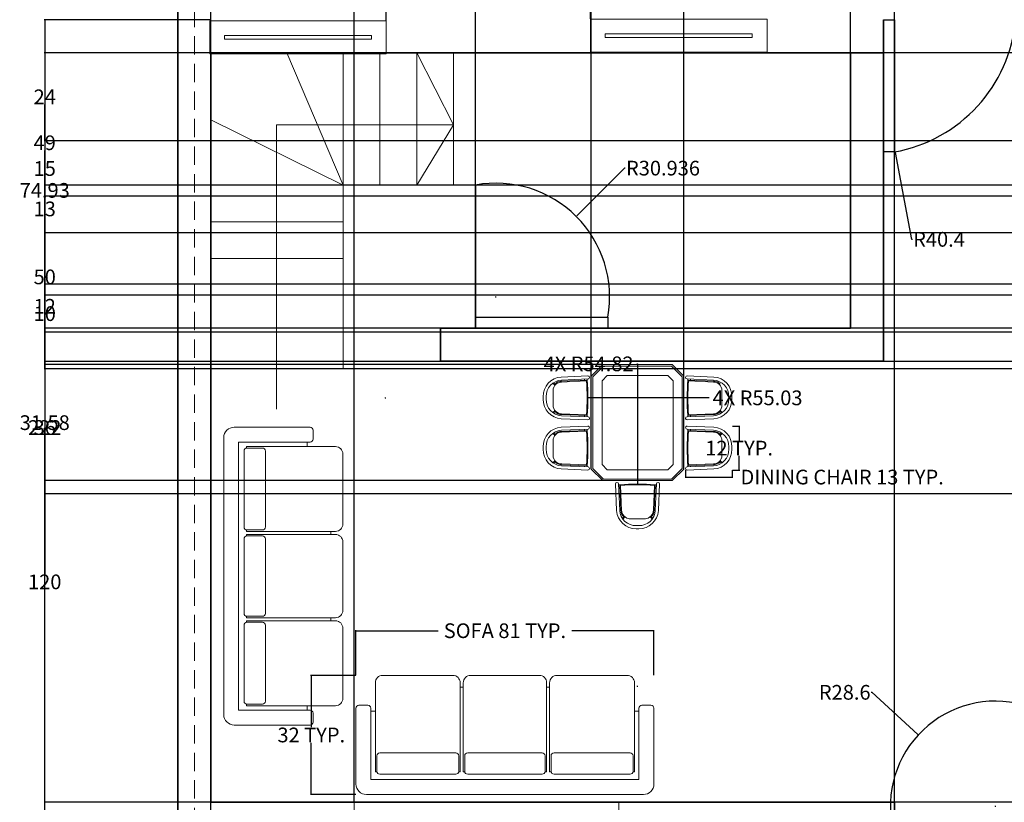
# Model space of a CAD drawing. Units: inches. Extents: x 1291 to 2095, y 532 to 1090.
# Tile 2 of 14: x 1291 to 1559, y 733 to 946. Entities that reach past the tile are written whole.
import ezdxf

# ---------------------------------------------------------------- set-up
doc = ezdxf.new("R2010")
doc.units = ezdxf.units.IN
doc.header["$MEASUREMENT"] = 0
doc.linetypes.add('HIDDEN', pattern=[0.375, 0.25, -0.125])
for name, color, linetype, lineweight in [('A-ANNO-DIMS', 2, 'Continuous', 18), ('A-DOOR', 3, 'Continuous', 25), ('A-FLOR-STRS', 7, 'Continuous', 20), ('A-FURN', 8, 'Continuous', 18), ('A-GLAZ', 4, 'Continuous', 18), ('A-WALL', 7, 'Continuous', 35), ('A-WALL-HIDN', 8, 'HIDDEN', 13)]:
    doc.layers.add(name, color=color, linetype=linetype, lineweight=lineweight)
doc.styles.get("Standard").update_dxf_attribs({"font": 'arial.ttf'})
doc.dimstyles.get("Standard").update_dxf_attribs({"dimtxt": 4, "dimasz": 0.18, "dimexe": 0.18, "dimexo": 0.0625, "dimgap": 0.09, "dimtad": 0, "dimtih": 1, "dimtoh": 1, "dimdec": 0, "dimrnd": 6, "dimzin": 0, "dimdsep": 46, "dimlunit": 3, "dimtxsty": 'Standard', "dimcen": 0.09, "dimadec": 0, "dimazin": 0, "dimtfac": 1, "dimtdec": 0, "dimtofl": 0, "dimtmove": 0, "dimatfit": 3, "dimfxl": 1, "dimtolj": 1, "dimtzin": 0, "dimarcsym": 0})

# ---------------------------------------------------------------- blocks, each defined once
blk = doc.blocks.new('A$C06FC73D7')
for p, q in [((1.93, 0.8), (0.07, 0.8)), ((0, 0.73), (0, 0.22)), ((2, 0.22), (2, 0.73)), ((0.1, 0.22), (0.1, 0.7)), ((0.1, 0.7), (1.9, 0.7)), ((0.67, 0.6637), (0.16, 0.6637)), ((1.25, 0.6637), (0.75, 0.6637)), ((1.84, 0.6637), (1.33, 0.6637)), ((1.9, 0.7), (1.9, 0.22)), ((0.13, 0.6479), (0.13, 0.05)), ((0.1404, 0.6479), (0.13, 0.6479)), ((0.14, 0.54), (0.14, 0.6437)), ((0.7, 0.6479), (0.6896, 0.6479)), ((0.69, 0.54), (0.69, 0.6437)), ((0.7, 0.05), (0.7, 0.6479)), ((0.72, 0.05), (0.72, 0.6479)), ((0.7304, 0.6479), (0.72, 0.6479)), ((0.73, 0.54), (0.73, 0.6437)), ((1.28, 0.6479), (1.2696, 0.6479)), ((1.27, 0.54), (1.27, 0.6437)), ((1.28, 0.05), (1.28, 0.6479)), ((1.3, 0.05), (1.3, 0.6479)), ((1.3104, 0.6479), (1.3, 0.6479)), ((1.31, 0.54), (1.31, 0.6437)), ((1.87, 0.6479), (1.86, 0.6479)), ((1.86, 0.54), (1.86, 0.6437)), ((1.87, 0.05), (1.87, 0.6479)), ((0.67, 0.52), (0.16, 0.52)), ((1.25, 0.52), (0.75, 0.52)), ((1.84, 0.52), (1.33, 0.52)), ((0.02, 0.2), (0.08, 0.2)), ((0.13, 0.24), (0.1, 0.24)), ((1.9, 0.24), (1.87, 0.24)), ((1.92, 0.2), (1.98, 0.2)), ((0.72, 0.08), (0.7, 0.08)), ((1.3, 0.08), (1.28, 0.08)), ((0.65, 0), (0.18, 0)), ((1.23, 0), (0.77, 0)), ((1.82, 0), (1.35, 0))]:
    blk.add_line(p, q)
for centre, radius, start, end in [((0.07, 0.73), 0.07, 90, 180), ((1.93, 0.73), 0.07, 0, 90), ((0.16, 0.6437), 0.02, 90, 180), ((0.67, 0.6437), 0.02, 0, 90), ((0.75, 0.6437), 0.02, 90, 180), ((1.25, 0.6437), 0.02, 0, 90), ((1.33, 0.6437), 0.02, 90, 180), ((1.84, 0.6437), 0.02, 0, 90), ((0.16, 0.54), 0.02, 180, 270), ((0.67, 0.54), 0.02, 270, 0), ((0.75, 0.54), 0.02, 180, 270), ((1.25, 0.54), 0.02, 270, 0), ((1.33, 0.54), 0.02, 180, 270), ((1.84, 0.54), 0.02, 270, 0), ((0.02, 0.22), 0.02, 180, 270), ((0.08, 0.22), 0.02, 270, 0), ((1.92, 0.22), 0.02, 180, 270), ((1.98, 0.22), 0.02, 270, 0), ((0.18, 0.05), 0.05, 180, 270), ((0.65, 0.05), 0.05, 270, 0), ((0.77, 0.05), 0.05, 180, 270), ((1.23, 0.05), 0.05, 270, 0), ((1.35, 0.05), 0.05, 180, 270), ((1.82, 0.05), 0.05, 270, 0)]:
    blk.add_arc(centre, radius, start, end)
blk = doc.blocks.new('A$C2BDD4447')
blk.add_blockref('A$C06FC73D7', (0, 0))
blk = doc.blocks.new('WIN-72IN')
for points in [[(0, 0), (0, 9), (72, 9), (72, 0)], [(4, 4), (4, 5), (68, 5), (68, 4)]]:
    blk.add_lwpolyline(points, close=True)
blk = doc.blocks.new('WIN-48IN')
for points in [[(0, 0), (0, 9), (48, 9), (48, 0)], [(4, 4), (4, 5), (44, 5), (44, 4)]]:
    blk.add_lwpolyline(points, close=True)
blk = doc.blocks.new('CHAIR-DINING')
for p, q in [((7.64, 10.83), (0.4, 11.13)), ((0.65, 11.13), (0.65, 10.81)), ((7.78, 10.51), (0.65, 10.8)), ((1.33, 11.1), (1.33, 10.78)), ((7.77, 10.3), (0.84, 10.59)), ((9.24, 9.6), (9.82, 10.09)), ((9.38, 9.44), (9.96, 9.93)), ((9.89, 3.77), (9.89, 8.24)), ((11.77, 5.65), (11.77, 6.32)), ((12.62, 5.64), (12.62, 6.33)), ((7.58, 1.45), (0.65, 1.16)), ((0.65, 0.84), (0.65, 1.15)), ((7.57, 1.66), (0.84, 1.38)), ((1.33, 0.87), (1.33, 1.18)), ((9.24, 2.37), (9.82, 1.88)), ((9.38, 2.53), (9.96, 2.04))]:
    blk.add_line(p, q)
for points in [[(7.68, 11.67), (0.44, 11.97, 1), (0.4, 11.13)], [(7.64, 1.14), (0.4, 0.84, 1), (0.44, 0), (7.68, 0.3)]]:
    blk.add_lwpolyline(points, format="xyb")
for centre, radius, start, end in [((55.47, 5.96), 55.03, 174.9478, 185.0066), ((7.37, 6.43), 4.41, 358.6114, 86.5609), ((7.37, 6.43), 5.25, 358.6113, 86.5608), ((55.47, 5.96), 54.82, 175.1561, 184.7886), ((7.58, 7.99), 2.52, 43.3469, 90), ((7.58, 7.99), 2.31, 0, 90), ((7.37, 5.54), 4.41, 273.4392, 1.3914), ((7.37, 5.54), 5.25, 273.4393, 1.3911), ((7.58, 3.97), 2.31, 270, 0), ((7.58, 3.97), 2.52, 270, 316.6497)]:
    blk.add_arc(centre, radius, start, end)
blk = doc.blocks.new('*D22')
at = {"layer": 'A-ANNO-DIMS', "color": 0, "lineweight": -2, "transparency": 16777216}
for p, q in [((1382.55, 767.39), (1382.55, 779.66)), ((1463.6, 767.39), (1463.6, 779.66)), ((1382.73, 779.48), (1404.87, 779.48)), ((1463.42, 779.48), (1441.27, 779.48))]:
    blk.add_line(p, q, dxfattribs=at)
at = {"layer": 'A-ANNO-DIMS', "color": 0, "transparency": 16777216}
for points in [[(1382.73, 779.51), (1382.73, 779.45), (1382.55, 779.48)], [(1463.42, 779.51), (1463.42, 779.45), (1463.6, 779.48)]]:
    blk.add_solid(points, dxfattribs=at)
at = {"layer": 'Defpoints', "color": 0, "transparency": 16777216}
for p in [(1382.55, 779.48), (1382.55, 767.33), (1463.6, 767.33)]:
    blk.add_point(p, dxfattribs=at)
at = {"layer": 'A-ANNO-DIMS', "color": 0, "transparency": 16777216, "insert": (1423.07, 779.48), "char_height": 4, "attachment_point": 5}
blk.add_mtext('\\A1;SOFA 81 TYP.', dxfattribs=at)
blk = doc.blocks.new('*D23')
at = {"layer": 'A-ANNO-DIMS', "color": 0, "lineweight": -2, "transparency": 16777216}
for p, q in [((1382.48, 767.33), (1370.21, 767.33)), ((1370.39, 767.15), (1370.39, 753.25)), ((1370.39, 735.08), (1370.39, 748.98)), ((1382.48, 734.9), (1370.21, 734.9))]:
    blk.add_line(p, q, dxfattribs=at)
at = {"layer": 'A-ANNO-DIMS', "color": 0, "transparency": 16777216}
for points in [[(1370.36, 767.15), (1370.42, 767.15), (1370.39, 767.33)], [(1370.36, 735.08), (1370.42, 735.08), (1370.39, 734.9)]]:
    blk.add_solid(points, dxfattribs=at)
at = {"layer": 'Defpoints', "color": 0, "transparency": 16777216}
for p in [(1382.55, 767.33), (1370.39, 734.9), (1382.55, 734.9)]:
    blk.add_point(p, dxfattribs=at)
at = {"layer": 'A-ANNO-DIMS', "color": 0, "transparency": 16777216, "insert": (1370.39, 751.11), "char_height": 4, "attachment_point": 5}
blk.add_mtext('\\A1;32 TYP.', dxfattribs=at)
blk = doc.blocks.new('*D24')
at = {"layer": 'A-ANNO-DIMS', "color": 0, "lineweight": -2, "transparency": 16777216}
for p, q in [((1472.2, 823.14), (1472.2, 821.12)), ((1484.89, 823.14), (1484.89, 821.12)), ((1472.38, 821.3), (1484.71, 821.3)), ((1484.89, 821.3), (1485.07, 821.3))]:
    blk.add_line(p, q, dxfattribs=at)
at = {"layer": 'A-ANNO-DIMS', "color": 0, "transparency": 16777216}
for points in [[(1472.38, 821.33), (1472.38, 821.27), (1472.2, 821.3)], [(1484.71, 821.33), (1484.71, 821.27), (1484.89, 821.3)]]:
    blk.add_solid(points, dxfattribs=at)
at = {"layer": 'Defpoints', "color": 0, "transparency": 16777216}
for p in [(1472.2, 823.2), (1484.89, 823.2), (1484.89, 821.3)]:
    blk.add_point(p, dxfattribs=at)
at = {"layer": 'A-ANNO-DIMS', "color": 0, "transparency": 16777216, "insert": (1514.82, 821.3), "char_height": 4, "attachment_point": 5}
blk.add_mtext('\\A1;DINING CHAIR 13 TYP.', dxfattribs=at)
blk = doc.blocks.new('*D25')
at = {"layer": 'A-ANNO-DIMS', "color": 0, "lineweight": -2, "transparency": 16777216}
for p, q in [((1484.95, 835.19), (1486.98, 835.19)), ((1486.8, 835.01), (1486.8, 831.29)), ((1486.8, 823.38), (1486.8, 827.09)), ((1484.95, 823.2), (1486.98, 823.2))]:
    blk.add_line(p, q, dxfattribs=at)
at = {"layer": 'A-ANNO-DIMS', "color": 0, "transparency": 16777216}
for points in [[(1486.77, 835.01), (1486.83, 835.01), (1486.8, 835.19)], [(1486.77, 823.38), (1486.83, 823.38), (1486.8, 823.2)]]:
    blk.add_solid(points, dxfattribs=at)
at = {"layer": 'Defpoints', "color": 0, "transparency": 16777216}
for p in [(1484.89, 835.19), (1486.8, 835.19), (1484.89, 823.2)]:
    blk.add_point(p, dxfattribs=at)
at = {"layer": 'A-ANNO-DIMS', "color": 0, "transparency": 16777216, "insert": (1486.8, 829.19), "char_height": 4, "attachment_point": 5}
blk.add_mtext('\\A1;12 TYP.', dxfattribs=at)
blk = doc.blocks.new('*D35')
at = {"layer": 'A-ANNO-DIMS', "color": 0, "lineweight": -2, "transparency": 16777216}
for p, q in [((1343.01, 945.78), (1297.69, 945.78)), ((1297.87, 945.6), (1297.87, 836.88)), ((1297.87, 723.96), (1297.87, 832.68)), ((1343.01, 723.78), (1297.69, 723.78))]:
    blk.add_line(p, q, dxfattribs=at)
at = {"layer": 'A-ANNO-DIMS', "color": 0, "transparency": 16777216}
for points in [[(1297.84, 945.6), (1297.9, 945.6), (1297.87, 945.78)], [(1297.84, 723.96), (1297.9, 723.96), (1297.87, 723.78)]]:
    blk.add_solid(points, dxfattribs=at)
at = {"layer": 'Defpoints', "color": 0, "transparency": 16777216}
for p in [(1297.87, 945.78), (1343.07, 945.78), (1343.07, 723.78)]:
    blk.add_point(p, dxfattribs=at)
at = {"layer": 'A-ANNO-DIMS', "color": 0, "transparency": 16777216, "insert": (1297.87, 834.78), "char_height": 4, "attachment_point": 5}
blk.add_mtext('\\A1;222', dxfattribs=at)
blk = doc.blocks.new('*D44')
at = {"layer": 'A-ANNO-DIMS', "color": 0, "lineweight": -2, "transparency": 16777216}
for p, q in [((1343.07, 579.84), (1343.07, 1087.16)), ((1343.25, 1086.98), (1451.42, 1086.98)), ((1576.43, 1086.98), (1468.26, 1086.98)), ((1576.61, 579.84), (1576.61, 1087.16))]:
    blk.add_line(p, q, dxfattribs=at)
at = {"layer": 'A-ANNO-DIMS', "color": 0, "transparency": 16777216}
for points in [[(1343.25, 1087.01), (1343.25, 1086.95), (1343.07, 1086.98)], [(1576.43, 1087.01), (1576.43, 1086.95), (1576.61, 1086.98)]]:
    blk.add_solid(points, dxfattribs=at)
at = {"layer": 'Defpoints', "color": 0, "transparency": 16777216}
for p in [(1576.61, 1086.98), (1343.07, 579.78), (1576.61, 579.78)]:
    blk.add_point(p, dxfattribs=at)
at = {"layer": 'A-ANNO-DIMS', "color": 0, "transparency": 16777216, "insert": (1459.84, 1086.98), "char_height": 4, "attachment_point": 5}
blk.add_mtext('\\A1;233.54', dxfattribs=at)
blk = doc.blocks.new('*D48')
at = {"layer": 'A-ANNO-DIMS', "color": 0, "lineweight": -2, "transparency": 16777216}
for p, q in [((1577.01, 852.78), (1297.69, 852.78)), ((1297.87, 852.6), (1297.87, 836.91)), ((1297.87, 816.96), (1297.87, 832.65)), ((1577.01, 816.78), (1297.69, 816.78))]:
    blk.add_line(p, q, dxfattribs=at)
at = {"layer": 'A-ANNO-DIMS', "color": 0, "transparency": 16777216}
for points in [[(1297.84, 852.6), (1297.9, 852.6), (1297.87, 852.78)], [(1297.84, 816.96), (1297.9, 816.96), (1297.87, 816.78)]]:
    blk.add_solid(points, dxfattribs=at)
at = {"layer": 'Defpoints', "color": 0, "transparency": 16777216}
for p in [(1297.87, 852.78), (1577.07, 852.78), (1577.07, 816.78)]:
    blk.add_point(p, dxfattribs=at)
at = {"layer": 'A-ANNO-DIMS', "color": 0, "transparency": 16777216, "insert": (1297.87, 834.78), "char_height": 4, "attachment_point": 5}
blk.add_mtext('\\A1;36', dxfattribs=at)
blk = doc.blocks.new('*D51')
at = {"layer": 'A-ANNO-DIMS', "color": 0, "lineweight": -2, "transparency": 16777216}
for p, q in [((1820.01, 852.78), (1297.69, 852.78)), ((1297.87, 852.6), (1297.87, 794.91)), ((1297.87, 732.96), (1297.87, 790.65)), ((1811.01, 732.78), (1297.69, 732.78))]:
    blk.add_line(p, q, dxfattribs=at)
at = {"layer": 'A-ANNO-DIMS', "color": 0, "transparency": 16777216}
for points in [[(1297.84, 852.6), (1297.9, 852.6), (1297.87, 852.78)], [(1297.84, 732.96), (1297.9, 732.96), (1297.87, 732.78)]]:
    blk.add_solid(points, dxfattribs=at)
at = {"layer": 'Defpoints', "color": 0, "transparency": 16777216}
for p in [(1297.87, 852.78), (1820.07, 852.78), (1811.07, 732.78)]:
    blk.add_point(p, dxfattribs=at)
at = {"layer": 'A-ANNO-DIMS', "color": 0, "transparency": 16777216, "insert": (1297.87, 792.78), "char_height": 4, "attachment_point": 5}
blk.add_mtext('\\A1;120', dxfattribs=at)
blk = doc.blocks.new('*D53')
at = {"layer": 'A-ANNO-DIMS', "color": 0, "lineweight": -2, "transparency": 16777216}
for p, q in [((1517, 936.78), (1297.69, 936.78)), ((1297.87, 936.6), (1297.87, 901.45)), ((1297.87, 862.03), (1297.87, 897.18)), ((1517, 861.85), (1297.69, 861.85))]:
    blk.add_line(p, q, dxfattribs=at)
at = {"layer": 'A-ANNO-DIMS', "color": 0, "transparency": 16777216}
for points in [[(1297.84, 936.6), (1297.9, 936.6), (1297.87, 936.78)], [(1297.84, 862.03), (1297.9, 862.03), (1297.87, 861.85)]]:
    blk.add_solid(points, dxfattribs=at)
at = {"layer": 'Defpoints', "color": 0, "transparency": 16777216}
for p in [(1297.87, 936.78), (1517.07, 936.78), (1517.07, 861.85)]:
    blk.add_point(p, dxfattribs=at)
at = {"layer": 'A-ANNO-DIMS', "color": 0, "transparency": 16777216, "insert": (1297.87, 899.32), "char_height": 4, "attachment_point": 5}
blk.add_mtext('\\A1;74.93', dxfattribs=at)
blk = doc.blocks.new('*D54')
at = {"layer": 'A-ANNO-DIMS', "color": 0, "lineweight": -2, "transparency": 16777216}
for p, q in [((1415.07, 861.91), (1415.07, 1087.16)), ((1415.25, 1086.98), (1461.77, 1086.98)), ((1516.89, 1086.98), (1470.37, 1086.98)), ((1517.07, 861.91), (1517.07, 1087.16))]:
    blk.add_line(p, q, dxfattribs=at)
at = {"layer": 'A-ANNO-DIMS', "color": 0, "transparency": 16777216}
for points in [[(1415.25, 1087.01), (1415.25, 1086.95), (1415.07, 1086.98)], [(1516.89, 1087.01), (1516.89, 1086.95), (1517.07, 1086.98)]]:
    blk.add_solid(points, dxfattribs=at)
at = {"layer": 'Defpoints', "color": 0, "transparency": 16777216}
for p in [(1517.07, 1086.98), (1415.07, 861.85), (1517.07, 861.85)]:
    blk.add_point(p, dxfattribs=at)
at = {"layer": 'A-ANNO-DIMS', "color": 0, "transparency": 16777216, "insert": (1466.07, 1086.98), "char_height": 4, "attachment_point": 5}
blk.add_mtext('\\A1;102', dxfattribs=at)
blk = doc.blocks.new('*D56')
at = {"layer": 'A-ANNO-DIMS', "color": 0, "lineweight": -2, "transparency": 16777216}
for p, q in [((1868.01, 936.78), (1297.69, 936.78)), ((1297.87, 936.6), (1297.87, 914.41)), ((1297.87, 887.96), (1297.87, 910.15)), ((1868.01, 887.78), (1297.69, 887.78))]:
    blk.add_line(p, q, dxfattribs=at)
at = {"layer": 'A-ANNO-DIMS', "color": 0, "transparency": 16777216}
for points in [[(1297.84, 936.6), (1297.9, 936.6), (1297.87, 936.78)], [(1297.84, 887.96), (1297.9, 887.96), (1297.87, 887.78)]]:
    blk.add_solid(points, dxfattribs=at)
at = {"layer": 'Defpoints', "color": 0, "transparency": 16777216}
for p in [(1297.87, 936.78), (1868.07, 936.78), (1868.07, 887.78)]:
    blk.add_point(p, dxfattribs=at)
at = {"layer": 'A-ANNO-DIMS', "color": 0, "transparency": 16777216, "insert": (1297.87, 912.28), "char_height": 4, "attachment_point": 5}
blk.add_mtext('\\A1;49', dxfattribs=at)
blk = doc.blocks.new('*D57')
at = {"layer": 'A-ANNO-DIMS', "color": 0, "lineweight": -2, "transparency": 16777216}
for p, q in [((1973.01, 900.78), (1297.69, 900.78)), ((1297.87, 900.6), (1297.87, 896.41)), ((1297.87, 887.96), (1297.87, 892.15)), ((1973.01, 887.78), (1297.69, 887.78))]:
    blk.add_line(p, q, dxfattribs=at)
at = {"layer": 'A-ANNO-DIMS', "color": 0, "transparency": 16777216}
for points in [[(1297.84, 900.6), (1297.9, 900.6), (1297.87, 900.78)], [(1297.84, 887.96), (1297.9, 887.96), (1297.87, 887.78)]]:
    blk.add_solid(points, dxfattribs=at)
at = {"layer": 'Defpoints', "color": 0, "transparency": 16777216}
for p in [(1297.87, 900.78), (1973.07, 900.78), (1973.07, 887.78)]:
    blk.add_point(p, dxfattribs=at)
at = {"layer": 'A-ANNO-DIMS', "color": 0, "transparency": 16777216, "insert": (1297.87, 894.28), "char_height": 4, "attachment_point": 5}
blk.add_mtext('\\A1;13', dxfattribs=at)
blk = doc.blocks.new('*D59')
at = {"layer": 'A-ANNO-DIMS', "color": 0, "lineweight": -2, "transparency": 16777216}
for p, q in [((2009.01, 900.78), (1297.69, 900.78)), ((1297.87, 900.6), (1297.87, 877.91)), ((1297.87, 850.96), (1297.87, 873.65)), ((2009.01, 850.78), (1297.69, 850.78))]:
    blk.add_line(p, q, dxfattribs=at)
at = {"layer": 'A-ANNO-DIMS', "color": 0, "transparency": 16777216}
for points in [[(1297.84, 900.6), (1297.9, 900.6), (1297.87, 900.78)], [(1297.84, 850.96), (1297.9, 850.96), (1297.87, 850.78)]]:
    blk.add_solid(points, dxfattribs=at)
at = {"layer": 'Defpoints', "color": 0, "transparency": 16777216}
for p in [(1297.87, 900.78), (2009.07, 900.78), (2009.07, 850.78)]:
    blk.add_point(p, dxfattribs=at)
at = {"layer": 'A-ANNO-DIMS', "color": 0, "transparency": 16777216, "insert": (1297.87, 875.78), "char_height": 4, "attachment_point": 5}
blk.add_mtext('\\A1;50', dxfattribs=at)
blk = doc.blocks.new('*D60')
at = {"layer": 'A-ANNO-DIMS', "color": 0, "lineweight": -2, "transparency": 16777216}
for p, q in [((2045.01, 870.78), (1297.69, 870.78)), ((1297.87, 870.6), (1297.87, 867.91)), ((1297.87, 860.96), (1297.87, 863.65)), ((2045.01, 860.78), (1297.69, 860.78))]:
    blk.add_line(p, q, dxfattribs=at)
at = {"layer": 'A-ANNO-DIMS', "color": 0, "transparency": 16777216}
for points in [[(1297.84, 870.6), (1297.9, 870.6), (1297.87, 870.78)], [(1297.84, 860.96), (1297.9, 860.96), (1297.87, 860.78)]]:
    blk.add_solid(points, dxfattribs=at)
at = {"layer": 'Defpoints', "color": 0, "transparency": 16777216}
for p in [(1297.87, 870.78), (2045.07, 870.78), (2045.07, 860.78)]:
    blk.add_point(p, dxfattribs=at)
at = {"layer": 'A-ANNO-DIMS', "color": 0, "transparency": 16777216, "insert": (1297.87, 865.78), "char_height": 4, "attachment_point": 5}
blk.add_mtext('\\A1;10', dxfattribs=at)
blk = doc.blocks.new('*D61')
at = {"layer": 'A-ANNO-DIMS', "color": 0, "lineweight": -2, "transparency": 16777216}
for p, q in [((1343.07, 732.84), (1343.07, 1087.16)), ((1343.25, 1086.98), (1355.7, 1086.98)), ((1381.84, 1086.98), (1369.4, 1086.98)), ((1382.02, 732.91), (1382.02, 1087.16))]:
    blk.add_line(p, q, dxfattribs=at)
at = {"layer": 'A-ANNO-DIMS', "color": 0, "transparency": 16777216}
for points in [[(1343.25, 1087.01), (1343.25, 1086.95), (1343.07, 1086.98)], [(1381.84, 1087.01), (1381.84, 1086.95), (1382.02, 1086.98)]]:
    blk.add_solid(points, dxfattribs=at)
at = {"layer": 'Defpoints', "color": 0, "transparency": 16777216}
for p in [(1382.02, 1086.98), (1343.07, 732.78), (1382.02, 732.85)]:
    blk.add_point(p, dxfattribs=at)
at = {"layer": 'A-ANNO-DIMS', "color": 0, "transparency": 16777216, "insert": (1362.55, 1086.98), "char_height": 4, "attachment_point": 5}
blk.add_mtext('\\A1;38.95', dxfattribs=at)
blk = doc.blocks.new('*D63')
at = {"layer": 'A-ANNO-DIMS', "color": 0, "lineweight": -2, "transparency": 16777216}
for p, q in [((1529.07, 723.84), (1529.07, 1087.16)), ((1529.25, 1086.98), (1544.12, 1086.98)), ((1564.89, 1086.98), (1550.03, 1086.98)), ((1565.07, 723.84), (1565.07, 1087.16))]:
    blk.add_line(p, q, dxfattribs=at)
at = {"layer": 'A-ANNO-DIMS', "color": 0, "transparency": 16777216}
for points in [[(1529.25, 1087.01), (1529.25, 1086.95), (1529.07, 1086.98)], [(1564.89, 1087.01), (1564.89, 1086.95), (1565.07, 1086.98)]]:
    blk.add_solid(points, dxfattribs=at)
at = {"layer": 'Defpoints', "color": 0, "transparency": 16777216}
for p in [(1565.07, 1086.98), (1529.07, 723.78), (1565.07, 723.78)]:
    blk.add_point(p, dxfattribs=at)
at = {"layer": 'A-ANNO-DIMS', "color": 0, "transparency": 16777216, "insert": (1547.07, 1086.98), "char_height": 4, "attachment_point": 5}
blk.add_mtext('\\A1;36', dxfattribs=at)
blk = doc.blocks.new('*D69')
at = {"layer": 'A-ANNO-DIMS', "color": 0, "lineweight": -2, "transparency": 16777216}
for p, q in [((1390.8, 945.53), (1390.8, 1087.16)), ((1390.98, 1086.98), (1411.75, 1086.98)), ((1446.2, 1086.98), (1425.43, 1086.98)), ((1446.38, 945.99), (1446.38, 1087.16))]:
    blk.add_line(p, q, dxfattribs=at)
at = {"layer": 'A-ANNO-DIMS', "color": 0, "transparency": 16777216}
for points in [[(1390.98, 1087.01), (1390.98, 1086.95), (1390.8, 1086.98)], [(1446.2, 1087.01), (1446.2, 1086.95), (1446.38, 1086.98)]]:
    blk.add_solid(points, dxfattribs=at)
at = {"layer": 'Defpoints', "color": 0, "transparency": 16777216}
for p in [(1446.38, 1086.98), (1446.38, 945.92), (1390.8, 945.47)]:
    blk.add_point(p, dxfattribs=at)
at = {"layer": 'A-ANNO-DIMS', "color": 0, "transparency": 16777216, "insert": (1418.59, 1086.98), "char_height": 4, "attachment_point": 5}
blk.add_mtext('\\A1;55.58', dxfattribs=at)
blk = doc.blocks.new('*D78')
at = {"layer": 'A-ANNO-DIMS', "color": 0, "lineweight": -2, "transparency": 16777216}
for p, q in [((1562.01, 936.78), (1297.69, 936.78)), ((1297.87, 936.6), (1297.87, 926.88)), ((1297.87, 912.96), (1297.87, 922.68)), ((1562.01, 912.78), (1297.69, 912.78))]:
    blk.add_line(p, q, dxfattribs=at)
at = {"layer": 'A-ANNO-DIMS', "color": 0, "transparency": 16777216}
for points in [[(1297.84, 936.6), (1297.9, 936.6), (1297.87, 936.78)], [(1297.84, 912.96), (1297.9, 912.96), (1297.87, 912.78)]]:
    blk.add_solid(points, dxfattribs=at)
at = {"layer": 'Defpoints', "color": 0, "transparency": 16777216}
for p in [(1297.87, 936.78), (1562.07, 936.78), (1562.07, 912.78)]:
    blk.add_point(p, dxfattribs=at)
at = {"layer": 'A-ANNO-DIMS', "color": 0, "transparency": 16777216, "insert": (1297.87, 924.78), "char_height": 4, "attachment_point": 5}
blk.add_mtext('\\A1;24', dxfattribs=at)
blk = doc.blocks.new('*D80')
at = {"layer": 'A-ANNO-DIMS', "color": 0, "lineweight": -2, "transparency": 16777216}
for p, q in [((1670.01, 912.78), (1297.69, 912.78)), ((1297.87, 912.6), (1297.87, 907.41)), ((1297.87, 897.96), (1297.87, 903.15)), ((1670.01, 897.78), (1297.69, 897.78))]:
    blk.add_line(p, q, dxfattribs=at)
at = {"layer": 'A-ANNO-DIMS', "color": 0, "transparency": 16777216}
for points in [[(1297.84, 912.6), (1297.9, 912.6), (1297.87, 912.78)], [(1297.84, 897.96), (1297.9, 897.96), (1297.87, 897.78)]]:
    blk.add_solid(points, dxfattribs=at)
at = {"layer": 'Defpoints', "color": 0, "transparency": 16777216}
for p in [(1297.87, 912.78), (1670.07, 912.78), (1670.07, 897.78)]:
    blk.add_point(p, dxfattribs=at)
at = {"layer": 'A-ANNO-DIMS', "color": 0, "transparency": 16777216, "insert": (1297.87, 905.28), "char_height": 4, "attachment_point": 5}
blk.add_mtext('\\A1;15', dxfattribs=at)
blk = doc.blocks.new('*D81')
at = {"layer": 'A-ANNO-DIMS', "color": 0, "lineweight": -2, "transparency": 16777216}
for p, q in [((1577.01, 873.78), (1297.69, 873.78)), ((1297.87, 873.6), (1297.87, 869.88)), ((1297.87, 861.96), (1297.87, 865.68)), ((1577.01, 861.78), (1297.69, 861.78))]:
    blk.add_line(p, q, dxfattribs=at)
at = {"layer": 'A-ANNO-DIMS', "color": 0, "transparency": 16777216}
for points in [[(1297.84, 873.6), (1297.9, 873.6), (1297.87, 873.78)], [(1297.84, 861.96), (1297.9, 861.96), (1297.87, 861.78)]]:
    blk.add_solid(points, dxfattribs=at)
at = {"layer": 'Defpoints', "color": 0, "transparency": 16777216}
for p in [(1297.87, 873.78), (1577.07, 873.78), (1577.07, 861.78)]:
    blk.add_point(p, dxfattribs=at)
at = {"layer": 'A-ANNO-DIMS', "color": 0, "transparency": 16777216, "insert": (1297.87, 867.78), "char_height": 4, "attachment_point": 5}
blk.add_mtext('\\A1;12', dxfattribs=at)
blk = doc.blocks.new('*D82')
at = {"layer": 'A-ANNO-DIMS', "color": 0, "lineweight": -2, "transparency": 16777216}
for p, q in [((1446.55, 823.54), (1446.55, 1087.16)), ((1446.73, 1086.98), (1450.72, 1086.98)), ((1471.56, 1086.98), (1467.57, 1086.98)), ((1471.74, 823.54), (1471.74, 1087.16))]:
    blk.add_line(p, q, dxfattribs=at)
at = {"layer": 'A-ANNO-DIMS', "color": 0, "transparency": 16777216}
for points in [[(1446.73, 1087.01), (1446.73, 1086.95), (1446.55, 1086.98)], [(1471.56, 1087.01), (1471.56, 1086.95), (1471.74, 1086.98)]]:
    blk.add_solid(points, dxfattribs=at)
at = {"layer": 'Defpoints', "color": 0, "transparency": 16777216}
for p in [(1471.74, 1086.98), (1446.55, 823.47), (1471.74, 823.47)]:
    blk.add_point(p, dxfattribs=at)
at = {"layer": 'A-ANNO-DIMS', "color": 0, "transparency": 16777216, "insert": (1459.15, 1086.98), "char_height": 4, "attachment_point": 5}
blk.add_mtext('\\A1;25.196', dxfattribs=at)
blk = doc.blocks.new('*D83')
at = {"layer": 'A-ANNO-DIMS', "color": 0, "lineweight": -2, "transparency": 16777216}
for p, q in [((1449.63, 851.9), (1297.69, 851.9)), ((1297.87, 851.72), (1297.87, 838.25)), ((1297.87, 820.5), (1297.87, 833.98)), ((1449.63, 820.32), (1297.69, 820.32))]:
    blk.add_line(p, q, dxfattribs=at)
at = {"layer": 'A-ANNO-DIMS', "color": 0, "transparency": 16777216}
for points in [[(1297.84, 851.72), (1297.9, 851.72), (1297.87, 851.9)], [(1297.84, 820.5), (1297.9, 820.5), (1297.87, 820.32)]]:
    blk.add_solid(points, dxfattribs=at)
at = {"layer": 'Defpoints', "color": 0, "transparency": 16777216}
for p in [(1297.87, 851.9), (1449.7, 851.9), (1449.7, 820.32)]:
    blk.add_point(p, dxfattribs=at)
at = {"layer": 'A-ANNO-DIMS', "color": 0, "transparency": 16777216, "insert": (1297.87, 836.11), "char_height": 4, "attachment_point": 5}
blk.add_mtext('\\A1;31.58', dxfattribs=at)
blk = doc.blocks.new('*D88')
at = {"layer": 'A-ANNO-DIMS', "color": 0, "lineweight": -2, "transparency": 16777216}
for p, q in [((1455.6, 905.38), (1442.61, 892.37)), ((1455.78, 905.38), (1455.6, 905.38)), ((1420.54, 870.35), (1420.72, 870.35)), ((1420.63, 870.26), (1420.63, 870.44))]:
    blk.add_line(p, q, dxfattribs=at)
at = {"layer": 'A-ANNO-DIMS', "color": 0, "transparency": 16777216}
blk.add_solid([(1442.59, 892.39), (1442.63, 892.35), (1442.48, 892.24)], dxfattribs=at)
at = {"layer": 'Defpoints', "color": 0, "transparency": 16777216}
for p in [(1442.48, 892.24), (1420.63, 870.35)]:
    blk.add_point(p, dxfattribs=at)
at = {"layer": 'A-ANNO-DIMS', "color": 0, "transparency": 16777216, "insert": (1466.08, 905.38), "char_height": 4, "attachment_point": 5}
blk.add_mtext('\\A1;R30.936', dxfattribs=at)
blk = doc.blocks.new('*D89')
at = {"layer": 'A-ANNO-DIMS', "color": 0, "lineweight": -2, "transparency": 16777216}
for p, q in [((1522.71, 762.72), (1522.89, 762.72)), ((1522.89, 762.72), (1535.38, 751.22)), ((1556.46, 731.72), (1556.64, 731.72)), ((1556.55, 731.63), (1556.55, 731.81))]:
    blk.add_line(p, q, dxfattribs=at)
at = {"layer": 'A-ANNO-DIMS', "color": 0, "transparency": 16777216}
blk.add_solid([(1535.4, 751.24), (1535.36, 751.2), (1535.51, 751.1)], dxfattribs=at)
at = {"layer": 'Defpoints', "color": 0, "transparency": 16777216}
for p in [(1535.51, 751.1), (1556.55, 731.72)]:
    blk.add_point(p, dxfattribs=at)
at = {"layer": 'A-ANNO-DIMS', "color": 0, "transparency": 16777216, "insert": (1515.52, 762.72), "char_height": 4, "attachment_point": 5}
blk.add_mtext('\\A1;R28.6', dxfattribs=at)
blk = doc.blocks.new('*D90')
at = {"layer": 'A-ANNO-DIMS', "color": 0, "lineweight": -2, "transparency": 16777216}
for p, q in [((1521.76, 949.52), (1521.94, 949.52)), ((1521.85, 949.43), (1521.85, 949.61)), ((1533.8, 886), (1529.35, 909.64)), ((1533.98, 886), (1533.8, 886))]:
    blk.add_line(p, q, dxfattribs=at)
at = {"layer": 'A-ANNO-DIMS', "color": 0, "transparency": 16777216}
blk.add_solid([(1529.38, 909.65), (1529.32, 909.63), (1529.32, 909.82)], dxfattribs=at)
at = {"layer": 'Defpoints', "color": 0, "transparency": 16777216}
for p in [(1521.85, 949.52), (1529.32, 909.82)]:
    blk.add_point(p, dxfattribs=at)
at = {"layer": 'A-ANNO-DIMS', "color": 0, "transparency": 16777216, "insert": (1541.17, 886), "char_height": 4, "attachment_point": 5}
blk.add_mtext('\\A1;R40.4', dxfattribs=at)
blk = doc.blocks.new('*D92')
at = {"layer": 'A-ANNO-DIMS', "color": 0, "lineweight": -2, "transparency": 16777216}
for p, q in [((1390.52, 842.82), (1390.7, 842.82)), ((1390.61, 842.73), (1390.61, 842.91)), ((1478.66, 842.86), (1445.82, 842.84))]:
    blk.add_line(p, q, dxfattribs=at)
at = {"layer": 'A-ANNO-DIMS', "color": 0, "transparency": 16777216}
blk.add_solid([(1445.82, 842.88), (1445.82, 842.82), (1445.64, 842.84)], dxfattribs=at)
at = {"layer": 'Defpoints', "color": 0, "transparency": 16777216}
for p in [(1390.61, 842.82), (1445.64, 842.84)]:
    blk.add_point(p, dxfattribs=at)
at = {"layer": 'A-ANNO-DIMS', "color": 0, "transparency": 16777216, "insert": (1491.8, 842.86), "char_height": 4, "attachment_point": 5}
blk.add_mtext('\\A1;4X R55.03', dxfattribs=at)
blk = doc.blocks.new('*D93')
at = {"layer": 'A-ANNO-DIMS', "color": 0, "lineweight": -2, "transparency": 16777216}
for p, q in [((1458.95, 852.11), (1459.13, 852.11)), ((1459.13, 852.11), (1459.15, 819.39)), ((1459.08, 764.39), (1459.26, 764.39)), ((1459.17, 764.3), (1459.17, 764.48))]:
    blk.add_line(p, q, dxfattribs=at)
at = {"layer": 'A-ANNO-DIMS', "color": 0, "transparency": 16777216}
blk.add_solid([(1459.18, 819.39), (1459.12, 819.39), (1459.15, 819.21)], dxfattribs=at)
at = {"layer": 'Defpoints', "color": 0, "transparency": 16777216}
for p in [(1459.15, 819.21), (1459.17, 764.39)]:
    blk.add_point(p, dxfattribs=at)
at = {"layer": 'A-ANNO-DIMS', "color": 0, "transparency": 16777216, "insert": (1445.84, 852.11), "char_height": 4, "attachment_point": 5}
blk.add_mtext('\\A1;4X R54.82', dxfattribs=at)

msp = doc.modelspace()

# ---------------------------------------------------------------- linework, layer by layer
at = {"layer": 'A-DOOR'}
for points in [[(1526.0658, 945.7707), (1529.0658, 945.7707), (1529.0658, 909.7707), (1526.0658, 909.7707)], [(1451.0735, 864.8516), (1451.0735, 861.8516), (1415.0735, 861.8516), (1415.0735, 864.8516)]]:
    msp.add_lwpolyline(points, close=True, dxfattribs=at)
for centre, radius, start, end in [((1521.8491, 949.5186), 40.3978, 280.290544, 354.690499), ((1420.6291, 870.3469), 30.9364, 349.767963, 100.345385), ((1556.5498, 731.7195), 28.6002, 78.580328, 196.116311)]:
    msp.add_arc(centre, radius, start, end, dxfattribs=at)
at = {"layer": 'A-FLOR-STRS'}
for p, q in [((1379.0735, 900.7804), (1363.7205, 936.7804)), ((1379.0735, 936.7804), (1379.0735, 850.7804)), ((1389.0735, 936.7804), (1389.0735, 900.7804)), ((1399.0735, 936.7804), (1399.0735, 900.7804)), ((1409.0735, 917.193), (1399.0735, 936.7804)), ((1409.0735, 936.7804), (1409.0735, 900.7804)), ((1415.0735, 936.7804), (1415.0735, 900.7804)), ((1379.0735, 900.7804), (1343.0735, 918.5024)), ((1360.9052, 839.8148), (1360.9052, 917.193)), ((1360.9052, 917.193), (1409.0735, 917.193)), ((1409.0735, 917.193), (1399.0735, 900.7804)), ((1415.0735, 900.7804), (1343.0735, 900.7804)), ((1379.0735, 890.7804), (1343.0735, 890.7804)), ((1379.0735, 880.7804), (1343.0735, 880.7804)), ((1379.0735, 870.7804), (1343.0735, 870.7804)), ((1379.0735, 860.7804), (1343.0735, 860.7804)), ((1379.0735, 850.7804), (1343.0735, 850.7804))]:
    msp.add_line(p, q, dxfattribs=at)
at = {"layer": 'A-FURN'}
for p, q in [((1436.7019, 846.3016), (1436.1232, 846.795)), ((1436.8382, 846.4613), (1436.2595, 846.9548)), ((1438.3016, 847.3741), (1445.4359, 847.6703)), ((1438.3147, 847.1643), (1445.2392, 847.4522)), ((1438.4453, 847.6941), (1445.6799, 847.9947)), ((1444.7499, 847.9649), (1444.7499, 847.6506)), ((1445.4351, 847.9947), (1445.4351, 847.6791)), ((1479.8459, 847.6941), (1472.6113, 847.9947)), ((1479.9895, 847.3741), (1472.8553, 847.6703)), ((1472.8561, 847.9947), (1472.8561, 847.6791)), ((1479.9765, 847.1643), (1473.052, 847.4522)), ((1473.5412, 847.9649), (1473.5412, 847.6506)), ((1436.1942, 840.6348), (1436.1942, 845.1016)), ((1482.097, 840.6348), (1482.097, 845.1016)), ((1433.4669, 842.5039), (1433.4669, 843.1947)), ((1434.3072, 842.5146), (1434.3072, 843.185)), ((1483.984, 842.5146), (1483.984, 843.185)), ((1484.8242, 842.5039), (1484.8242, 843.1947)), ((1436.7019, 839.3983), (1436.1232, 838.9046)), ((1436.8382, 839.2385), (1436.2595, 838.745)), ((1438.5099, 838.5273), (1445.2438, 838.2474)), ((1479.7813, 838.5273), (1473.0474, 838.2474)), ((1481.453, 839.2385), (1482.0317, 838.745)), ((1481.5893, 839.3983), (1482.168, 838.9046)), ((1438.5059, 838.3173), (1445.4357, 838.0293)), ((1444.7499, 837.7349), (1444.7499, 838.049)), ((1445.4351, 837.7049), (1445.4351, 838.0207)), ((1479.7852, 838.3173), (1472.8555, 838.0293)), ((1472.8561, 837.7049), (1472.8561, 838.0207)), ((1473.5412, 837.7349), (1473.5412, 838.049)), ((1454.3014, 812.2219), (1454.0008, 819.4565)), ((1454.0008, 819.2117), (1454.3163, 819.2117)), ((1454.0306, 818.5266), (1454.3449, 818.5266)), ((1454.6214, 812.0783), (1454.3252, 819.2126)), ((1454.8312, 812.0913), (1454.5433, 819.0158)), ((1463.4682, 812.2866), (1463.7481, 819.0204)), ((1463.6781, 812.2826), (1463.9662, 819.2123)), ((1464.2606, 818.5266), (1463.9465, 818.5266)), ((1464.2906, 819.2117), (1463.9748, 819.2117)), ((1455.5341, 810.6148), (1455.0407, 810.0361)), ((1455.6939, 810.4786), (1455.2005, 809.8999)), ((1461.3607, 809.9708), (1456.8939, 809.9708)), ((1462.5972, 810.4786), (1463.0909, 809.8999)), ((1462.757, 810.6148), (1463.2504, 810.0361)), ((1459.4916, 807.2436), (1458.8008, 807.2436)), ((1459.4809, 808.0839), (1458.8105, 808.0839))]:
    msp.add_line(p, q, dxfattribs=at)
for points in [[(1471.7436, 823.4737), (1471.7436, 848.7533), (1468.5941, 851.9028), (1449.6971, 851.9028), (1446.5476, 848.7533), (1446.5476, 823.4737), (1449.6971, 820.3242), (1468.5941, 820.3242)], [(1471.3237, 848.5793), (1471.3237, 823.6352), (1468.4327, 820.7441), (1449.8833, 820.7441), (1446.9862, 823.6413), (1446.9675, 848.5793), (1449.8711, 851.4829), (1468.4203, 851.4829)], [(1468.8041, 847.5357), (1468.8041, 824.6913), (1467.3765, 823.2638), (1450.9147, 823.2638), (1449.4871, 824.6913), (1449.4871, 847.5357), (1450.9147, 848.9633), (1467.3765, 848.9633)]]:
    msp.add_lwpolyline(points, close=True, dxfattribs=at)
for points in [[(1445.6799, 847.9945, 1), (1445.645, 848.834), (1438.4018, 848.5329)], [(1479.8894, 848.5329), (1472.6462, 848.834, 1), (1472.6113, 847.9945)], [(1438.4018, 837.1669), (1445.645, 836.8658, 1), (1445.6799, 837.7049), (1438.4453, 838.0058)], [(1479.8459, 838.0058), (1472.6113, 837.7049, 1), (1472.6462, 836.8658), (1479.8894, 837.1669)], [(1454.001, 819.4565, 1), (1453.1615, 819.4217), (1453.4626, 812.1784)], [(1464.8286, 812.1784), (1465.1296, 819.4217, 1), (1464.2906, 819.4565), (1463.9897, 812.2219)]]:
    msp.add_lwpolyline(points, format="xyb", dxfattribs=at)
for centre, radius, start, end in [((1438.7161, 843.2921), 5.2501, 93.439216, 181.388744), ((1438.7161, 843.2921), 4.4102, 93.439136, 181.388601), ((1438.5062, 844.8606), 2.3119, 90, 180), ((1438.5062, 844.8606), 2.5218, 90, 136.653148), ((1390.6114, 842.8234), 54.8236, 355.211394, 4.843878), ((1390.6114, 842.8234), 55.0335, 354.993413, 5.052231), ((1527.6798, 842.8234), 55.0335, 174.947769, 185.006587), ((1527.6798, 842.8234), 54.8236, 175.156122, 184.788606), ((1479.785, 844.8606), 2.5218, 43.346852, 90), ((1479.785, 844.8606), 2.3119, 0, 90), ((1479.5751, 843.2921), 4.4102, 358.611399, 86.560864), ((1479.5751, 843.2921), 5.2501, 358.611256, 86.560784), ((1438.7161, 842.4075), 5.25, 178.608948, 266.560743), ((1438.7161, 842.4075), 4.4101, 178.608646, 266.560815), ((1479.5751, 842.4075), 4.4101, 273.439185, 1.391354), ((1479.5751, 842.4075), 5.25, 273.439257, 1.391052), ((1438.5062, 840.8393), 2.3119, 180, 270), ((1438.5062, 840.8393), 2.5219, 223.350321, 270), ((1479.785, 840.8393), 2.3119, 270, 0), ((1479.785, 840.8393), 2.5219, 270, 316.649679), ((1459.172, 764.388), 55.0335, 84.993413, 95.052231), ((1459.172, 764.388), 54.8236, 85.211394, 94.843878), ((1458.7034, 812.4928), 5.2501, 183.439216, 271.388744), ((1458.7034, 812.4928), 4.4102, 183.439136, 271.388601), ((1457.1349, 812.2828), 2.5218, 180, 226.653148), ((1457.1349, 812.2828), 2.3119, 180, 270), ((1459.588, 812.4928), 5.25, 268.608948, 356.560743), ((1459.588, 812.4928), 4.4101, 268.608646, 356.560815), ((1461.1562, 812.2828), 2.3119, 270, 0), ((1461.1562, 812.2828), 2.5219, 313.350321, 0)]:
    msp.add_arc(centre, radius, start, end, dxfattribs=at)
at = {"layer": 'A-WALL'}
for p, q in [((1334.0735, 1050.7804), (1334.0735, 570.7804)), ((1526.0735, 936.7804), (1526.0735, 945.7804)), ((1526.0735, 936.7804), (1343.0735, 936.7804)), ((1343.0735, 936.7804), (1343.0735, 732.7804)), ((1517.0658, 936.7804), (1517.0658, 861.8516)), ((1526.0658, 936.7804), (1526.0658, 852.8516)), ((1415.0735, 900.7804), (1415.0735, 861.8516)), ((1405.5816, 861.8516), (1517.0658, 861.8516)), ((1405.5816, 861.8516), (1405.5816, 852.8516)), ((1405.5816, 852.8516), (1526.0658, 852.8516)), ((1343.0735, 732.7804), (1529.0735, 732.7804)), ((1529.0735, 723.7804), (1529.0735, 732.7804))]:
    msp.add_line(p, q, dxfattribs=at)
at = {"layer": 'A-WALL-HIDN', "ltscale": 20}
msp.add_line((1338.5735, 1046.2804), (1338.5735, 570.7804), dxfattribs=at)

# ---------------------------------------------------------------- block references
at = {"layer": 'A-FURN', "xscale": 40.52616843532049, "yscale": 40.52616843532049, "zscale": 40.52616843532049}
for p, rotation in [((1378.9933, 753.8148), 90), ((1463.5993, 767.3251), 180)]:
    msp.add_blockref('A$C2BDD4447', p, dxfattribs=dict(at, rotation=rotation))
at = {"layer": 'A-FURN', "extrusion": (0, 0, -1), "zscale": -1}
msp.add_blockref('CHAIR-DINING', (-1446.0822, 823.209), dxfattribs=at)
at = {"layer": 'A-FURN'}
msp.add_blockref('CHAIR-DINING', (1472.209, 823.209), dxfattribs=at)
at = {"layer": 'A-GLAZ'}
for name, p in [('WIN-48IN', (1446.3793, 936.9233)), ('WIN-48IN', (1342.7982, 936.4703)), ('WIN-72IN', (1382.0238, 723.8457))]:
    msp.add_blockref(name, p, dxfattribs=at)

# ---------------------------------------------------------------- dimensions: what is measured, and where the dimension line sits
at = {"layer": 'A-ANNO-DIMS'}
for base, p1, p2, override, picture, middle in [((1576.6107, 1086.9804), (1343.0735, 579.7804), (1576.6107, 579.7804), {"dimdec": 2, "dimlfac": 1, "dimrnd": 0, "dimzin": 0, "dimdsep": 46, "dimlunit": 2}, '*D44', (1459.8421, 1086.9804)), ((1382.0234, 1086.9804), (1343.0735, 732.7804), (1382.0234, 732.8453), {"dimdec": 2, "dimlfac": 1, "dimrnd": 0, "dimzin": 0, "dimdsep": 46, "dimlunit": 2}, '*D61', (1362.5485, 1086.9804)), ((1446.3797, 1086.9804), (1390.7986, 945.4707), (1446.3797, 945.9238), {"dimdec": 2, "dimlfac": 1, "dimrnd": 0, "dimzin": 0, "dimdsep": 46, "dimlunit": 2}, '*D69', (1418.5892, 1086.9804)), ((1517.0658, 1086.9804), (1415.0735, 861.8516), (1517.0658, 861.8516), {"dimdec": 0, "dimlfac": 1, "dimrnd": 0, "dimzin": 0, "dimdsep": 46, "dimlunit": 2}, '*D54', (1466.0697, 1086.9804)), ((1471.7436, 1086.9804), (1446.5476, 823.4737), (1471.7436, 823.4737), {"dimdec": 3, "dimlfac": 1, "dimrnd": 0, "dimzin": 0, "dimdsep": 46, "dimlunit": 2}, '*D82', (1459.1456, 1086.9804)), ((1565.0735, 1086.9804), (1529.0735, 723.7804), (1565.0735, 723.7804), {"dimdec": 0, "dimlfac": 1, "dimrnd": 0, "dimzin": 0, "dimdsep": 46, "dimlunit": 2}, '*D63', (1547.0735, 1086.9804))]:
    dim = msp.add_linear_dim(base=base, p1=p1, p2=p2, dimstyle='Standard', override=override, dxfattribs=at)
    dim.commit()
    dim.dimension.update_dxf_attribs({"geometry": picture, "text_midpoint": middle})
for center, mpoint, override, picture, middle in [((1521.8491, 949.5186), (1529.3156, 909.8169), {"dimdec": 1, "dimlfac": 1, "dimrnd": 0, "dimzin": 0, "dimdsep": 46, "dimlunit": 2}, '*D90', (1541.1665, 885.9958)), ((1420.62914, 870.34694), (1442.48287, 892.24387), {"dimdec": 3, "dimlfac": 1, "dimrnd": 0, "dimzin": 0, "dimdsep": 46, "dimlunit": 2}, '*D88', (1466.08065, 905.38202)), ((1556.5498, 731.7195), (1535.5147, 751.0973), {"dimdec": 1, "dimlfac": 1, "dimrnd": 0, "dimzin": 0, "dimdsep": 46, "dimlunit": 2}, '*D89', (1515.5159, 762.724))]:
    dim = msp.add_radius_dim(center=center, mpoint=mpoint, dimstyle='Standard', override=override, dxfattribs=at)
    dim.commit()
    dim.dimension.update_dxf_attribs({"geometry": picture, "text_midpoint": middle, "dimtype": 164})
for base, p1, p2, override, picture, middle in [((1297.8735, 945.7804), (1343.0735, 723.7804), (1343.0735, 945.7804), {"dimdec": 0, "dimlfac": 1, "dimrnd": 0, "dimzin": 0, "dimdsep": 46, "dimlunit": 2}, '*D35', (1297.8735, 834.7804)), ((1297.8735, 936.7804), (1517.0658, 861.8516), (1517.0658, 936.7804), {"dimdec": 2, "dimlfac": 1, "dimrnd": 0, "dimzin": 0, "dimdsep": 46, "dimlunit": 2}, '*D53', (1297.8735, 899.316)), ((1297.8735, 936.7804), (1868.0735, 887.7804), (1868.0735, 936.7804), {"dimdec": 0, "dimlfac": 1, "dimrnd": 0, "dimzin": 0, "dimdsep": 46, "dimlunit": 2}, '*D56', (1297.8735, 912.2804)), ((1297.8735, 936.7804), (1562.0735, 912.7804), (1562.0735, 936.7804), {"dimdec": 0, "dimlfac": 1, "dimrnd": 0, "dimzin": 0, "dimdsep": 46, "dimlunit": 2}, '*D78', (1297.8735, 924.7804)), ((1297.8735, 912.7804), (1670.0735, 897.7804), (1670.0735, 912.7804), {"dimdec": 0, "dimlfac": 1, "dimrnd": 0, "dimzin": 0, "dimdsep": 46, "dimlunit": 2}, '*D80', (1297.8735, 905.2804)), ((1297.8735, 900.7804), (1973.0735, 887.7804), (1973.0735, 900.7804), {"dimdec": 0, "dimlfac": 1, "dimrnd": 0, "dimzin": 0, "dimdsep": 46, "dimlunit": 2}, '*D57', (1297.8735, 894.2804)), ((1297.8735, 900.7804), (2009.0735, 850.7804), (2009.0735, 900.7804), {"dimdec": 0, "dimlfac": 1, "dimrnd": 0, "dimzin": 0, "dimdsep": 46, "dimlunit": 2}, '*D59', (1297.8735, 875.7804)), ((1297.8735, 873.7804), (1577.0735, 861.7804), (1577.0735, 873.7804), {"dimdec": 0, "dimlfac": 1, "dimrnd": 0, "dimzin": 0, "dimdsep": 46, "dimlunit": 2}, '*D81', (1297.8735, 867.7804)), ((1297.8735, 870.7804), (2045.0735, 860.7804), (2045.0735, 870.7804), {"dimdec": 0, "dimlfac": 1, "dimrnd": 0, "dimzin": 0, "dimdsep": 46, "dimlunit": 2}, '*D60', (1297.8735, 865.7804)), ((1297.8735, 851.9028), (1449.6971, 820.3242), (1449.6971, 851.9028), {"dimdec": 2, "dimlfac": 1, "dimrnd": 0, "dimzin": 0, "dimdsep": 46, "dimlunit": 2}, '*D83', (1297.8735, 836.1135)), ((1297.8735, 852.7804), (1811.0735, 732.7804), (1820.0735, 852.7804), {"dimdec": 0, "dimlfac": 1, "dimrnd": 0, "dimzin": 0, "dimdsep": 46, "dimlunit": 2}, '*D51', (1297.8735, 792.7804)), ((1297.8735, 852.7804), (1577.0735, 816.7804), (1577.0735, 852.7804), {"dimdec": 0, "dimlfac": 1, "dimrnd": 0, "dimzin": 0, "dimdsep": 46, "dimlunit": 2}, '*D48', (1297.8735, 834.7804))]:
    dim = msp.add_linear_dim(base=base, p1=p1, p2=p2, angle=90, dimstyle='Standard', override=override, dxfattribs=at)
    dim.commit()
    dim.dimension.update_dxf_attribs({"geometry": picture, "text_midpoint": middle})
for center, mpoint, picture, middle in [((1459.172, 764.388), (1459.146, 819.2116), '*D93', (1445.8399, 852.1058)), ((1390.6114, 842.8234), (1445.6449, 842.845), '*D92', (1478.665, 842.8579))]:
    dim = msp.add_radius_dim(center=center, mpoint=mpoint, text='4X <>', dimstyle='Standard', override={"dimdec": 2, "dimlfac": 1, "dimrnd": 0, "dimzin": 0, "dimdsep": 46, "dimlunit": 2}, dxfattribs=at)
    dim.commit()
    dim.dimension.update_dxf_attribs({"geometry": picture, "text_midpoint": middle, "dimtype": 164})
dim = msp.add_linear_dim(base=(1484.8922, 821.2953), p1=(1472.1994, 823.1993), p2=(1484.8922, 823.1993), text='DINING CHAIR <> TYP.', dimstyle='Standard', override={"dimdec": 0, "dimlfac": 1, "dimrnd": 0, "dimzin": 0, "dimdsep": 46, "dimlunit": 2}, dxfattribs=at)
dim.commit()
dim.dimension.update_dxf_attribs({"geometry": '*D24', "text_midpoint": (1514.8225, 821.2953)})
for base, p1, p2, angle, text, picture, middle in [((1486.7961, 835.1866), (1484.8922, 823.1993), (1484.8922, 835.1866), 90, '<> TYP.', '*D25', (1486.7961, 829.193)), ((1382.5469, 779.483), (1463.5993, 767.3251), (1382.5469, 767.3251), 180, 'SOFA <> TYP.', '*D22', (1423.0731, 779.483)), ((1370.3891, 734.9042), (1382.5469, 767.3251), (1382.5469, 734.9042), 270, '<> TYP.', '*D23', (1370.3891, 751.1147))]:
    dim = msp.add_linear_dim(base=base, p1=p1, p2=p2, angle=angle, text=text, dimstyle='Standard', override={"dimdec": 0, "dimlfac": 1, "dimrnd": 0, "dimzin": 0, "dimdsep": 46, "dimlunit": 2}, dxfattribs=at)
    dim.commit()
    dim.dimension.update_dxf_attribs({"geometry": picture, "text_midpoint": middle})

doc.saveas('drawing.dxf')
